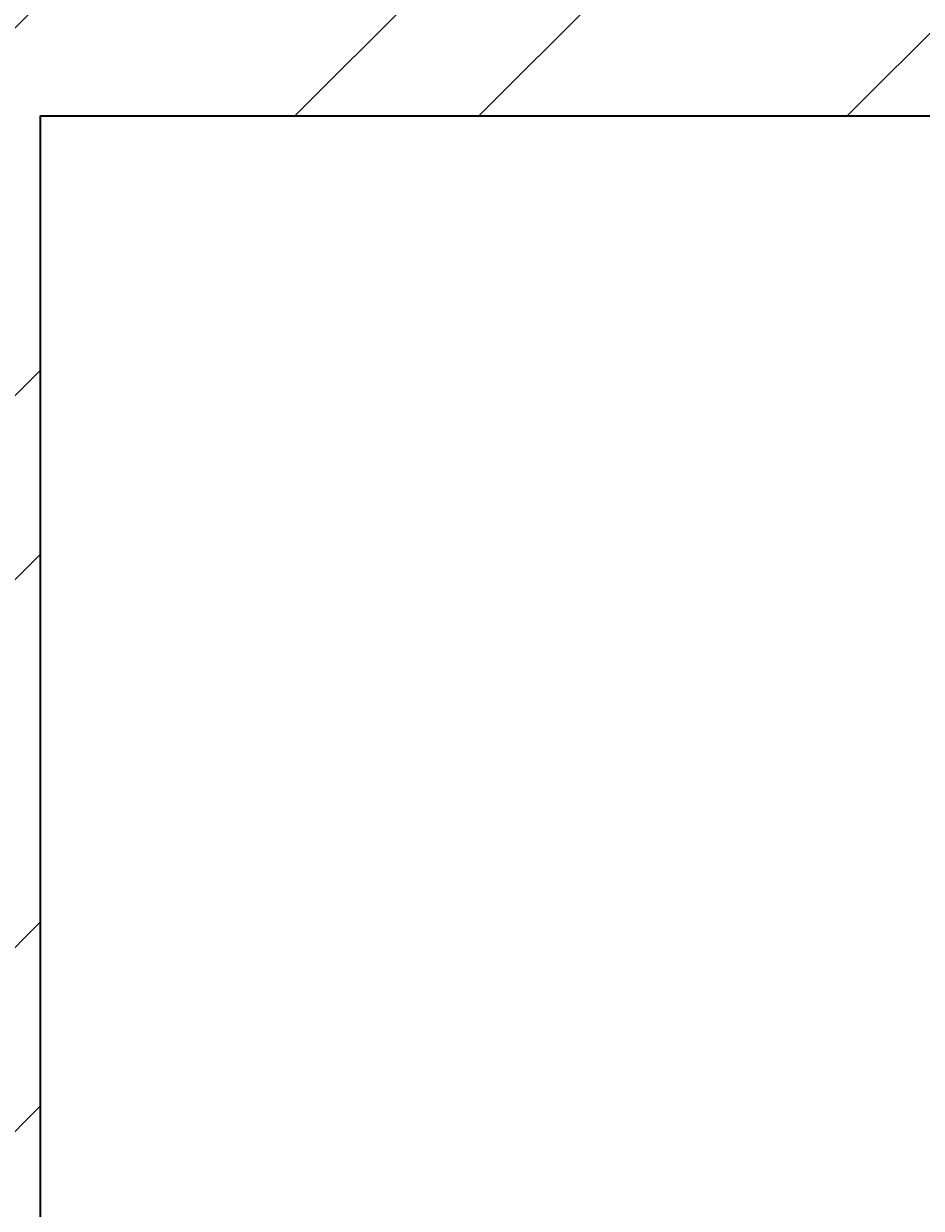
# Model space of a CAD drawing. Units: inches. Extents: x 1962 to 2771, y 1245 to 2660.
# Tile 49 of 114: x 2090 to 2112, y 2151 to 2180. Entities that reach past the tile are written whole.
import ezdxf

# ---------------------------------------------------------------- set-up
doc = ezdxf.new("R2010")
doc.units = ezdxf.units.IN
for name, color, linetype, lineweight in [('A-ANNO-DIMS', 2, 'Continuous', 18), ('A-WALL', 7, 'Continuous', 35), ('A-WALL-PATT', 252, 'Continuous', 13)]:
    doc.layers.add(name, color=color, linetype=linetype, lineweight=lineweight)
doc.styles.get("Standard").update_dxf_attribs({"font": 'arial.ttf'})
doc.dimstyles.get("Standard").update_dxf_attribs({"dimtxt": 0.18, "dimasz": 0.18, "dimexe": 0.18, "dimexo": 0.0625, "dimgap": 0.09, "dimtad": 0, "dimtih": 1, "dimtoh": 1, "dimdec": 4, "dimzin": 0, "dimdsep": 46, "dimtxsty": 'Standard', "dimcen": 0.09, "dimadec": 0, "dimazin": 0, "dimtfac": 1, "dimtdec": 4, "dimtofl": 0, "dimtmove": 0, "dimatfit": 3, "dimfxl": 1, "dimtolj": 1, "dimtzin": 0, "dimarcsym": 0})

# ---------------------------------------------------------------- blocks, each defined once
blk = doc.blocks.new('*D40')
at = {"layer": 'A-ANNO-DIMS', "color": 0, "lineweight": -2, "transparency": 16777216}
for p, q in [((2072.02, 2033.906), (2072.02, 2583.474)), ((2072.2, 2583.294), (2366.02, 2583.294)), ((2660.627, 2583.294), (2366.808, 2583.294)), ((2660.807, 2524.406), (2660.807, 2583.474))]:
    blk.add_line(p, q, dxfattribs=at)
at = {"layer": 'A-ANNO-DIMS', "color": 0, "transparency": 16777216}
for points in [[(2072.2, 2583.324), (2072.2, 2583.264), (2072.02, 2583.294)], [(2660.627, 2583.324), (2660.627, 2583.264), (2660.807, 2583.294)]]:
    blk.add_solid(points, dxfattribs=at)
at = {"layer": 'Defpoints', "color": 0, "transparency": 16777216}
for p in [(2660.807, 2583.294), (2660.807, 2524.344), (2072.02, 2033.844)]:
    blk.add_point(p, dxfattribs=at)
at = {"layer": 'A-ANNO-DIMS', "color": 0, "transparency": 16777216, "insert": (2366.414, 2583.294), "char_height": 0.18, "attachment_point": 5}
blk.add_mtext('\\A1;588.8', dxfattribs=at)

msp = doc.modelspace()

# ---------------------------------------------------------------- hatches: boundary and pattern name
at = {"layer": 'A-WALL-PATT'}
h = msp.add_hatch(dxfattribs=at)
h.set_pattern_fill('ANSI32', color=256)
h.paths.add_polyline_path([(2090.8074, 2467.3437), (2141.6481, 2467.3437), (2141.6481, 2469.5937), (2141.6481, 2471.8437), (2086.3074, 2471.8437), (2086.3074, 2422.5333), (2090.8074, 2422.5333)])
h.paths.add_polyline_path([(2282.7664, 2471.8437), (2204.8982, 2471.8437), (2204.8982, 2467.3437), (2234.8074, 2467.3437), (2234.8074, 2311.3437), (2228.7492, 2311.3437), (2228.7492, 2306.8437), (2234.8074, 2306.8437), (2331.9227, 2306.8437), (2331.9227, 2309.0937), (2331.9227, 2311.3437), (2239.3074, 2311.3437), (2239.3074, 2467.3437), (2282.7664, 2467.3437), (2282.7664, 2469.5937)])
h.paths.add_polyline_path([(2471.4531, 2519.8437), (2552.011, 2519.8437), (2564.3996, 2519.8437), (2564.3996, 2511.1389), (2568.8996, 2511.1389), (2568.8996, 2524.3437), (2466.9531, 2524.3437), (2466.9531, 2471.8437), (2450.0749, 2471.8437), (2446.4672, 2471.8437), (2446.4672, 2467.3437), (2450.0749, 2467.3437), (2475.9988, 2467.3437), (2475.9988, 2469.5937), (2475.9988, 2471.8437), (2471.4531, 2471.8437)])
h.paths.add_polyline_path([(2575.2231, 2469.5937), (2575.2231, 2471.8437), (2568.8996, 2471.8437), (2568.8996, 2487.1389), (2564.3996, 2487.1389), (2564.3996, 2471.8437), (2556.511, 2471.8437), (2499.2904, 2471.8437), (2499.2904, 2467.3437), (2507.8074, 2467.3437), (2507.8074, 2311.3437), (2414.863, 2311.3437), (2414.863, 2306.8437), (2512.3074, 2306.8437), (2517.0114, 2306.8437), (2517.0114, 2309.0937), (2517.0114, 2311.3437), (2512.3074, 2311.3437), (2512.3074, 2467.3437), (2575.2231, 2467.3437)])
h.paths.add_polyline_path([(2660.8074, 2471.8437), (2600.9602, 2471.8437), (2600.9602, 2467.3437), (2656.3074, 2467.3437), (2656.3074, 2432.5704), (2660.8074, 2432.5704)])
h.paths.add_polyline_path([(2660.8074, 2372.5704), (2656.3074, 2372.5704), (2656.3074, 2311.3437), (2600.276, 2311.3437), (2600.276, 2309.0937), (2600.276, 2306.8437), (2656.3074, 2306.8437), (2656.3074, 2296.2593), (2660.8074, 2296.2593)])
h.paths.add_polyline_path([(2572.3074, 2306.8437), (2577.1385, 2306.8437), (2577.1385, 2311.3437), (2551.082, 2311.3437), (2551.082, 2306.8437), (2567.8074, 2306.8437), (2567.8074, 2258.8437), (2540.0574, 2258.8437), (2540.0574, 2256.5937), (2540.0574, 2254.3437), (2567.8074, 2254.3437), (2656.3074, 2254.3437), (2656.3074, 2236.9085), (2660.8074, 2236.9085), (2660.8074, 2272.2593), (2656.3074, 2272.2593), (2656.3074, 2258.8437), (2572.3074, 2258.8437)])
h.paths.add_polyline_path([(2512.3074, 2254.3437), (2518.8716, 2254.3437), (2518.8716, 2256.5937), (2518.8716, 2258.8437), (2507.8074, 2258.8437), (2507.8074, 2177.8437), (2567.8074, 2177.8437), (2567.8074, 2172.9628), (2572.3074, 2172.9628), (2572.3074, 2177.8437), (2656.3074, 2177.8437), (2656.3074, 2166.4846), (2660.8074, 2166.4846), (2660.8074, 2200.9085), (2656.3074, 2200.9085), (2656.3074, 2182.3437), (2512.3074, 2182.3437)])
h.paths.add_polyline_path([(2656.3074, 2129.8437), (2572.3074, 2129.8437), (2572.3074, 2150.3044), (2570.0574, 2150.3044), (2567.8074, 2150.3044), (2567.8074, 2129.8437), (2507.8074, 2129.8437), (2507.8074, 2116.3027), (2510.0574, 2116.3027), (2512.3074, 2116.3027), (2512.3074, 2125.3437), (2567.8074, 2125.3437), (2572.3074, 2125.3437), (2656.3074, 2125.3437)])
h.paths.add_polyline_path([(2090.8074, 2362.5333), (2086.3074, 2362.5333), (2086.3074, 2298.6242), (2090.8074, 2298.6242), (2090.8074, 2306.8437), (2174.8074, 2306.8437), (2174.8074, 2286.4178), (2179.3074, 2286.4178), (2179.3074, 2306.8437), (2192.8641, 2306.8437), (2192.8641, 2309.0937), (2192.8641, 2311.3437), (2090.8074, 2311.3437)])
h.paths.add_polyline_path([(2209.156, 2258.8437), (2179.3074, 2258.8437), (2179.3074, 2263.2236), (2177.0574, 2263.2236), (2174.8074, 2263.2236), (2174.8074, 2258.8437), (2090.8074, 2258.8437), (2090.8074, 2274.6242), (2086.3074, 2274.6242), (2086.3074, 2238.2967), (2088.5574, 2238.2967), (2090.8074, 2238.2967), (2090.8074, 2254.3437), (2209.156, 2254.3437)])
h.paths.add_polyline_path([(2090.8074, 2177.8437), (2234.8074, 2177.8437), (2234.8074, 2173.1428), (2239.3074, 2173.1428), (2239.3074, 2258.8437), (2230.8442, 2258.8437), (2230.8442, 2256.5937), (2230.8442, 2254.3437), (2234.8074, 2254.3437), (2234.8074, 2182.3437), (2090.8074, 2182.3437), (2090.8074, 2202.2967), (2086.3074, 2202.2967), (2086.3074, 2140.0389), (2090.8074, 2140.0389)])
h.paths.add_polyline_path([(2090.8074, 2080.0389), (2086.3074, 2080.0389), (2086.3074, 2033.8437), (2090.8074, 2033.8437)], flags=17)
h.paths.add_polyline_path([(2244.9405, 2033.8437), (2239.3074, 2033.8437), (2239.3074, 2142.0665), (2237.2592, 2142.0665), (2234.8074, 2142.0665), (2234.8074, 2033.8437), (2090.8074, 2033.8437), (2076.5204, 2033.8437), (2072.0204, 2033.8437), (2072.0204, 2000.4493), (2076.5204, 2000.4493), (2076.5204, 2029.3437), (2090.8074, 2029.3437), (2244.9405, 2029.3437), (2244.9405, 2031.5937)])
h.paths.add_polyline_path([(2234.8074, 1933.3437), (2076.5204, 1933.3437), (2076.5204, 1952.4493), (2074.2704, 1952.4493), (2072.0204, 1952.4493), (2072.0204, 1933.3437), (2072.0204, 1928.8437), (2234.8074, 1928.8437)])
h.paths.add_polyline_path([(2090.8074, 1928.8437), (2086.3074, 1928.8437), (2086.3074, 1906.5013), (2090.8074, 1906.5013)])
h.paths.add_polyline_path([(2090.8074, 1846.5013), (2086.3074, 1846.5013), (2086.3074, 1769.9917), (2088.5574, 1769.9917), (2090.8074, 1769.9917), (2090.8074, 1780.3437), (2234.8074, 1780.3437), (2234.8074, 1708.3437), (2230.3764, 1708.3437), (2230.3764, 1703.8437), (2239.3074, 1703.8437), (2239.3074, 1792.6669), (2237.0574, 1792.6669), (2234.8074, 1792.6669), (2234.8074, 1784.8437), (2090.8074, 1784.8437)])
h.paths.add_polyline_path([(2239.3074, 1928.8437), (2244.9405, 1928.8437), (2244.9405, 1931.0937), (2244.9405, 1933.3437), (2234.8074, 1933.3437), (2234.8074, 1928.8437), (2234.8074, 1825.5949), (2239.3074, 1825.5949)])
h.paths.add_polyline_path([(2148.0425, 1649.0937), (2148.0425, 1651.3437), (2090.8074, 1651.3437), (2090.8074, 1646.8437), (2148.0425, 1646.8437)], flags=0)
h.paths.add_polyline_path([(2207.5601, 1708.3437), (2090.8074, 1708.3437), (2090.8074, 1703.8437), (2174.8074, 1703.8437), (2174.8074, 1651.3437), (2170.4457, 1651.3437), (2170.4457, 1646.8437), (2195.9924, 1646.8437), (2195.9924, 1649.0937), (2195.9924, 1651.3437), (2179.3074, 1651.3437), (2179.3074, 1703.8437), (2207.5601, 1703.8437), (2207.5601, 1706.0937)])
h.paths.add_polyline_path([(2090.8074, 1733.9917), (2086.3074, 1733.9917), (2086.3074, 1696.1032), (2088.5574, 1696.1032), (2090.8074, 1696.1032)])
h.paths.add_polyline_path([(2090.8074, 1672.1032), (2086.3074, 1672.1032), (2086.3074, 1600.3335), (2090.8074, 1600.3335)])
h.paths.add_polyline_path([(2090.8074, 1540.3335), (2086.3074, 1540.3335), (2086.3074, 1486.3437), (2139.6766, 1486.3437), (2139.6766, 1490.8437), (2090.8074, 1490.8437)])
h.paths.add_polyline_path([(2302.3876, 1490.8437), (2239.3074, 1490.8437), (2239.3074, 1646.8437), (2335.9994, 1646.8437), (2335.9994, 1651.3437), (2229.884, 1651.3437), (2229.884, 1646.8437), (2234.8074, 1646.8437), (2234.8074, 1490.8437), (2202.7103, 1490.8437), (2202.7103, 1488.5937), (2202.7103, 1486.3437), (2275.0699, 1486.3437), (2275.0699, 1475.772), (2279.5699, 1475.772), (2279.5699, 1486.3437), (2302.3876, 1486.3437)])
h.paths.add_polyline_path([(2279.5699, 1451.772), (2275.0699, 1451.772), (2275.0699, 1438.3437), (2174.8074, 1438.3437), (2174.8074, 1486.3437), (2179.7922, 1486.3437), (2179.7922, 1490.8437), (2163.3585, 1490.8437), (2163.3585, 1488.5937), (2163.3585, 1486.3437), (2170.3074, 1486.3437), (2170.3074, 1433.8437), (2279.5699, 1433.8437)])
h.paths.add_polyline_path([(2427.2363, 1490.8437), (2375.8074, 1490.8437), (2375.8074, 1646.8437), (2381.6401, 1646.8437), (2381.6401, 1651.3437), (2365.887, 1651.3437), (2365.887, 1649.0937), (2365.887, 1646.8437), (2371.3074, 1646.8437), (2371.3074, 1490.8437), (2327.5627, 1490.8437), (2327.5627, 1488.5937), (2327.5627, 1486.3437), (2371.3074, 1486.3437), (2371.3074, 1433.8437), (2375.8074, 1433.8437), (2375.8074, 1486.3437), (2427.2363, 1486.3437)])
h.paths.add_polyline_path([(2512.3074, 1646.8437), (2519.4351, 1646.8437), (2519.4351, 1649.0937), (2519.4351, 1651.3437), (2507.8074, 1651.3437), (2416.0063, 1651.3437), (2416.0063, 1649.0937), (2416.0063, 1646.8437), (2507.8074, 1646.8437), (2507.8074, 1490.8437), (2497.0532, 1490.8437), (2497.0532, 1488.5937), (2497.0532, 1486.3437), (2574.9344, 1486.3437), (2574.9344, 1476.0181), (2579.4344, 1476.0181), (2579.4344, 1486.3437), (2584.4872, 1486.3437), (2584.3074, 1490.8437), (2512.3074, 1490.8437)])
h.paths.add_polyline_path([(2470.5091, 1486.3437), (2473.9767, 1486.3437), (2473.9767, 1490.8437), (2449.6605, 1490.8437), (2449.6605, 1488.5937), (2449.6605, 1486.3437), (2466.0091, 1486.3437), (2466.0091, 1433.8437), (2470.5091, 1433.8437), (2579.4344, 1433.8437), (2579.4344, 1452.0181), (2574.9344, 1452.0181), (2574.9344, 1438.3437), (2554.5091, 1438.3437), (2470.5091, 1438.3437)])
h.paths.add_polyline_path([(2656.3074, 1490.8437), (2611.86, 1490.8437), (2611.86, 1486.3437), (2656.3074, 1486.3437)])
h.paths.add_polyline_path([(2660.8074, 1532.7007), (2658.5574, 1532.7007), (2656.3074, 1532.7007), (2656.3074, 1486.3437), (2660.8074, 1486.3437)])
h.paths.add_polyline_path([(2660.8074, 1664.9663), (2656.3074, 1664.9663), (2656.3074, 1651.3437), (2602.2313, 1651.3437), (2602.2313, 1646.8437), (2656.3074, 1646.8437), (2656.3074, 1592.7007), (2660.8074, 1592.7007)])
h.paths.add_polyline_path([(2660.8074, 1724.5221), (2656.3074, 1724.5221), (2656.3074, 1703.8437), (2542.4725, 1703.8437), (2542.4725, 1699.3437), (2567.8074, 1699.3437), (2567.8074, 1651.3437), (2552.7766, 1651.3437), (2552.7766, 1649.0937), (2552.7766, 1646.8437), (2577.2878, 1646.8437), (2577.2878, 1649.0937), (2577.2878, 1651.3437), (2572.3074, 1651.3437), (2572.3074, 1699.3437), (2656.3074, 1699.3437), (2656.3074, 1688.9663), (2660.8074, 1688.9663)])
h.paths.add_polyline_path([(2660.8074, 1880.6524), (2656.3074, 1880.6524), (2656.3074, 1832.8437), (2512.3074, 1832.8437), (2512.3074, 1837.8959), (2507.8074, 1837.8959), (2507.8074, 1828.3437), (2567.8074, 1828.3437), (2567.8074, 1804.3437), (2572.3074, 1804.3437), (2572.3074, 1828.3437), (2656.3074, 1828.3437), (2656.3074, 1818.6778), (2660.8074, 1818.6778)])
h.paths.add_polyline_path([(2660.8074, 1794.6778), (2656.3074, 1794.6778), (2656.3074, 1780.3437), (2572.3074, 1780.3437), (2572.3074, 1783.0303), (2570.0574, 1783.0303), (2567.8074, 1783.0303), (2567.8074, 1780.3437), (2507.8074, 1780.3437), (2507.8074, 1699.3437), (2517.8858, 1699.3437), (2517.8858, 1701.5937), (2517.8858, 1703.8437), (2512.3074, 1703.8437), (2512.3074, 1775.8437), (2656.3074, 1775.8437), (2656.3074, 1760.5221), (2660.8074, 1760.5221)])
h.paths.add_polyline_path([(2660.8074, 1981.3437), (2660.8074, 2020.2808), (2658.5574, 2020.2808), (2656.3074, 2020.2808), (2656.3074, 1981.3437), (2512.3074, 1981.3437), (2512.3074, 2086.6996), (2507.8074, 2086.6996), (2507.8074, 1981.3437), (2375.8074, 1981.3437), (2375.8074, 1986.8505), (2373.5574, 1986.8505), (2371.3074, 1986.8505), (2371.3074, 1973.2607), (2375.8074, 1973.2607), (2375.8074, 1976.8437), (2507.8074, 1976.8437), (2507.8074, 1865.4281), (2510.0574, 1865.4281), (2512.3074, 1865.4281), (2512.3074, 1976.8437), (2660.8074, 1976.8437)])
h.paths.add_polyline_path([(2375.8074, 1940.297), (2373.5574, 1940.297), (2371.3074, 1940.297), (2371.3074, 1933.3437), (2278.4434, 1933.3437), (2278.4434, 1928.8437), (2371.3074, 1928.8437), (2371.3074, 1651.3437), (2375.8074, 1651.3437)])
h.paths.add_polyline_path([(2660.8074, 1976.8437), (2656.3074, 1976.8437), (2656.3074, 1940.6524), (2660.8074, 1940.6524)], flags=17)
h.paths.add_polyline_path([(2660.8074, 2142.4846), (2656.3074, 2142.4846), (2656.3074, 2080.2808), (2660.8074, 2080.2808)])
h.paths.add_polyline_path([(2381.4189, 2311.3437), (2375.8074, 2311.3437), (2375.8074, 2467.3437), (2424.7242, 2467.3437), (2424.7242, 2469.5937), (2424.7242, 2471.8437), (2375.8074, 2471.8437), (2375.8074, 2524.3437), (2371.3074, 2524.3437), (2371.3074, 2471.8437), (2307.2097, 2471.8437), (2307.2097, 2467.3437), (2371.3074, 2467.3437), (2371.3074, 2311.3437), (2366.8901, 2311.3437), (2366.8901, 2306.8437), (2371.3074, 2306.8437), (2371.3074, 2033.8437), (2279.6589, 2033.8437), (2279.6589, 2029.3437), (2371.3074, 2029.3437), (2371.3074, 2014.2598), (2375.8074, 2014.2598), (2375.8074, 2306.8437), (2381.4189, 2306.8437)])
h.paths.add_polyline_path([(2263.3074, 2524.3437), (2170.3074, 2524.3437), (2170.3074, 2519.8437), (2170.3074, 2471.8437), (2165.0312, 2471.8437), (2165.0312, 2467.3437), (2179.6721, 2467.3437), (2179.6721, 2469.5161), (2179.6721, 2471.8437), (2174.8074, 2471.8437), (2174.8074, 2519.8437), (2258.8074, 2519.8437), (2258.8074, 2511.6436), (2263.3074, 2511.6436)])
h.paths.add_polyline_path([(2245.0232, 1361.4123), (2492.9468, 1361.4123), (2492.9468, 1398.505), (2245.0232, 1398.505)], flags=9)
h.paths.add_polyline_path([(2388.1434, 2086.6936), (2425.0704, 2086.6936), (2425.0704, 2105.3509), (2388.1434, 2105.3509)], flags=9)
h.paths.add_polyline_path([(2404.922, 2242.6744), (2445.7337, 2242.6744), (2445.7337, 2261.3318), (2404.922, 2261.3318)], flags=9)
h.paths.add_polyline_path([(2269.4107, 2156.7935), (2306.3378, 2156.7935), (2306.3378, 2175.4508), (2269.4107, 2175.4508)], flags=9)
h.paths.add_polyline_path([(2269.3277, 2233.4343), (2306.2547, 2233.4343), (2306.2547, 2252.0917), (2269.3277, 2252.0917)], flags=9)
h.paths.add_polyline_path([(2431.6052, 2320.6922), (2470.4456, 2320.6922), (2470.4456, 2339.3495), (2431.6052, 2339.3495)], flags=25)
h.paths.add_polyline_path([(2249.6902, 2315.7608), (2288.5306, 2315.7608), (2288.5306, 2334.4182), (2249.6902, 2334.4182)], flags=25)
h.paths.add_polyline_path([(2096.9301, 2314.3181), (2135.7704, 2314.3181), (2135.7704, 2332.9755), (2096.9301, 2332.9755)], flags=25)
h.paths.add_polyline_path([(2134.3475, 2285.7089), (2161.4655, 2285.7089), (2161.4655, 2304.3662), (2134.3475, 2304.3662)], flags=9)
h.paths.add_polyline_path([(2126.5155, 2209.4076), (2159.9227, 2209.4076), (2159.9227, 2228.065), (2126.5155, 2228.065)], flags=25)
h.paths.add_polyline_path([(2110.5753, 2141.5299), (2149.4157, 2141.5299), (2149.4157, 2160.1872), (2110.5753, 2160.1872)], flags=25)
h.paths.add_polyline_path([(2249.8618, 1968.3317), (2286.3966, 1968.3317), (2286.3966, 1986.989), (2249.8618, 1986.989)], flags=9)
h.paths.add_polyline_path([(2395.9507, 1777.0051), (2436.7624, 1777.0051), (2436.7624, 1795.6625), (2395.9507, 1795.6625)], flags=9)
h.paths.add_polyline_path([(2398.5259, 1888.5651), (2435.0062, 1888.5651), (2435.0062, 1907.2224), (2398.5259, 1907.2224)], flags=25)
h.paths.add_polyline_path([(2259.3506, 1728.3559), (2296.2776, 1728.3559), (2296.2776, 1747.0132), (2259.3506, 1747.0132)], flags=9)
h.paths.add_polyline_path([(2271.3698, 1845.268), (2308.2968, 1845.268), (2308.2968, 1863.9253), (2271.3698, 1863.9253)], flags=9)
h.paths.add_polyline_path([(2120.9355, 1786.3027), (2159.7759, 1786.3027), (2159.7759, 1804.9601), (2120.9355, 1804.9601)], flags=25)
h.paths.add_polyline_path([(2121.3164, 1732.1043), (2154.7236, 1732.1043), (2154.7236, 1750.7616), (2121.3164, 1750.7616)], flags=25)
h.paths.add_polyline_path([(2118.3706, 1678.8997), (2147.5282, 1678.8997), (2147.5282, 1697.557), (2118.3706, 1697.557)], flags=25)
h.paths.add_polyline_path([(2385.9227, 1493.557), (2424.763, 1493.557), (2424.763, 1512.2143), (2385.9227, 1512.2143)], flags=25)
h.paths.add_polyline_path([(2248.7058, 1500.0256), (2287.5462, 1500.0256), (2287.5462, 1518.6829), (2248.7058, 1518.6829)], flags=25)
h.paths.add_polyline_path([(2104.1669, 1617.3771), (2143.0073, 1617.3771), (2143.0073, 1636.0344), (2104.1669, 1636.0344)], flags=9)
h.paths.add_polyline_path([(2096.0714, 1447.8824), (2137.3845, 1447.8824), (2137.3845, 1458.1859), (2096.0714, 1458.1859)], flags=9)
h.paths.add_polyline_path([(2180.6114, 1440.325), (2209.7689, 1440.325), (2209.7689, 1458.9823), (2180.6114, 1458.9823)], flags=25)
h.paths.add_polyline_path([(2316.1698, 1447.9637), (2357.4829, 1447.9637), (2357.4829, 1458.2673), (2316.1698, 1458.2673)], flags=9)
h.paths.add_polyline_path([(2397.6187, 1447.9637), (2438.9318, 1447.9637), (2438.9318, 1458.2673), (2397.6187, 1458.2673)], flags=9)
h.paths.add_polyline_path([(2473.0778, 1439.5953), (2502.2354, 1439.5953), (2502.2354, 1458.2527), (2473.0778, 1458.2527)], flags=25)
h.paths.add_polyline_path([(2589.7027, 1447.8819), (2631.0158, 1447.8819), (2631.0158, 1458.1855), (2589.7027, 1458.1855)], flags=9)
h.paths.add_polyline_path([(2522.4009, 1497.5285), (2561.2413, 1497.5285), (2561.2413, 1516.1859), (2522.4009, 1516.1859)], flags=25)
h.paths.add_polyline_path([(2579.6565, 1671.3482), (2608.8141, 1671.3482), (2608.8141, 1690.0056), (2579.6565, 1690.0056)], flags=25)
h.paths.add_polyline_path([(2544.7038, 1725.5064), (2578.1111, 1725.5064), (2578.1111, 1744.1637), (2544.7038, 1744.1637)], flags=25)
h.paths.add_polyline_path([(2578.1191, 1807.472), (2607.2766, 1807.472), (2607.2766, 1826.1293), (2578.1191, 1826.1293)], flags=25)
h.paths.add_polyline_path([(2595.0614, 1835.1839), (2633.9018, 1835.1839), (2633.9018, 1853.8413), (2595.0614, 1853.8413)], flags=25)
h.paths.add_polyline_path([(2567.0097, 2097.7035), (2605.8501, 2097.7035), (2605.8501, 2116.3609), (2567.0097, 2116.3609)], flags=9)
h.paths.add_polyline_path([(2586.644, 2134.6454), (2615.8015, 2134.6454), (2615.8015, 2153.3027), (2586.644, 2153.3027)], flags=9)
h.paths.add_polyline_path([(2544.6185, 2212.6783), (2578.0258, 2212.6783), (2578.0258, 2231.3356), (2544.6185, 2231.3356)], flags=25)
h.paths.add_polyline_path([(2577.0273, 2256.9023), (2606.1849, 2256.9023), (2606.1849, 2275.5597), (2577.0273, 2275.5597)], flags=24)
h.paths.add_polyline_path([(2605.2683, 2315.2821), (2644.1087, 2315.2821), (2644.1087, 2333.9395), (2605.2683, 2333.9395)], flags=25)
h.paths.add_polyline_path([(2583.1244, 2496.1815), (2624.4375, 2496.1815), (2624.4375, 2506.4851), (2583.1244, 2506.4851)], flags=9)
h.paths.add_polyline_path([(2474.761, 2497.0823), (2503.9185, 2497.0823), (2503.9185, 2515.7397), (2474.761, 2515.7397)], flags=25)
h.paths.add_polyline_path([(2387.5787, 2494.2563), (2428.902, 2494.2563), (2428.902, 2504.5598), (2387.5787, 2504.5598)], flags=9)
h.paths.add_polyline_path([(2300.1657, 2500.1564), (2341.4788, 2500.1564), (2341.4788, 2510.46), (2300.1657, 2510.46)], flags=25)
h.paths.add_polyline_path([(2176.8589, 2497.5843), (2206.0165, 2497.5843), (2206.0165, 2516.2416), (2176.8589, 2516.2416)], flags=25)
h.paths.add_polyline_path([(2097.4668, 2494.9762), (2138.7799, 2494.9762), (2138.7799, 2505.2798), (2097.4668, 2505.2798)], flags=9)

# ---------------------------------------------------------------- linework, layer by layer
at = {"layer": 'A-WALL'}
for q in [(2234.8074, 2177.8437), (2090.8074, 2033.8437)]:
    msp.add_line((2090.8074, 2177.8437), q, dxfattribs=at)

# ---------------------------------------------------------------- dimensions: what is measured, and where the dimension line sits
at = {"layer": 'A-ANNO-DIMS'}
dim = msp.add_linear_dim(base=(2660.8074, 2583.2937), p1=(2072.0204, 2033.8437), p2=(2660.8074, 2524.3437), dimstyle='Standard', override={"dimdec": 1, "dimlfac": 1, "dimrnd": 0, "dimzin": 0, "dimdsep": 46, "dimlunit": 2}, dxfattribs=at)
dim.commit()
dim.dimension.update_dxf_attribs({"geometry": '*D40', "text_midpoint": (2366.4139, 2583.2937)})

doc.saveas('drawing.dxf')
